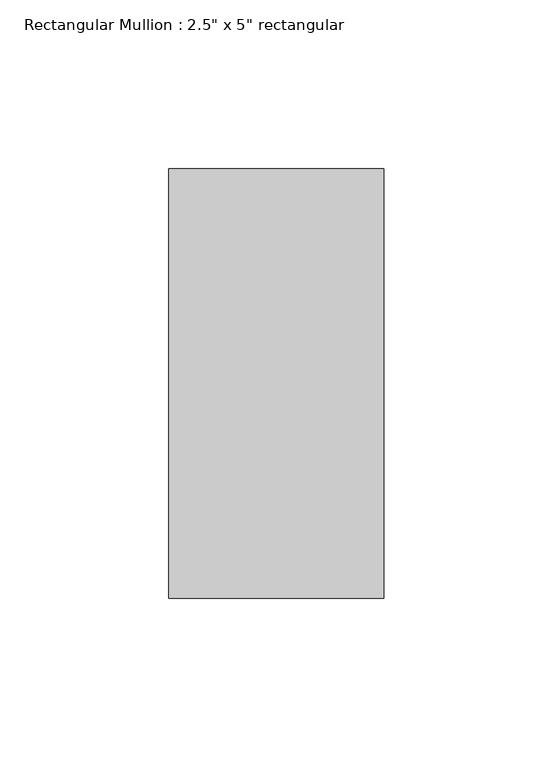
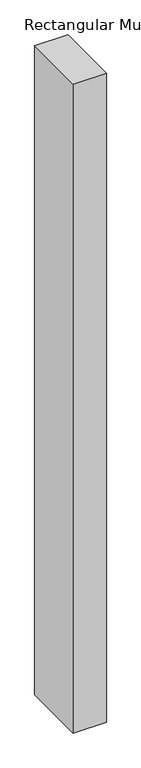
"""IFC4 building model written with IfcOpenShell, lengths in millimetres: member geometry."""

from ifc_helpers import new_model, si_unit, frame, origin, place, context, project, spatial, polyline, outline, extrude, source, transform, mapped, element, save


def member_c0a82454(model_context):
    return source(origin(), model_context, "Body", "SweptSolid", [
        extrude(outline(polyline([(0.0, 63.5), (0.0, -63.5), (-63.5, -63.5), (-63.5, 63.5), (0.0, 63.5)])), frame((0.0, 0.0, -1310.2166668), z_axis=(0.0, 0.0, 1.0), x_axis=(1.0, 0.0, 0.0)), (0.0, 0.0, 1.0), 1310.2166668),
    ])


if __name__ == "__main__":
    model = new_model("IFC4")
    model_context = context("Model", 3, world=origin())
    ifc_project = project(units=[si_unit("LENGTHUNIT", "METRE", prefix="MILLI")], contexts=[model_context])
    site = spatial("IfcSite", under=ifc_project)
    building = spatial("IfcBuilding", under=site)
    placement = place(None, origin())
    member_shape = member_c0a82454(model_context)
    element("IfcMember", 1, ObjectType="Rectangular Mullion : 2.5\" x 5\" rectangular", at=placement, inside=building, context=model_context, shape_type="MappedRepresentation", body=[
        mapped(member_shape, transform((0.0, 0.0, 0.0), x_axis=(1.0, 0.0, 0.0), y_axis=(0.0, 1.0, 0.0), z_axis=(0.0, 0.0, 1.0))),
    ])
    save(model, "model.ifc")

# Revit data of these elements
# Type "Rectangular Mullion : 2.5\" x 5\" rectangular"
#   built-in parameter 1007304 = 0.416667 (stored number, unit not read)
#   built-in parameter 1007301 = 0.104167 (stored number, unit not read)
#   built-in parameter 1007300 = 0.104167 (stored number, unit not read)
# Element 1 (IfcMember, "Rectangular Mullion : 2.5\" x 5\" rectangular")
#   Materials on its faces: "Aluminum"
# Materials
#   "Aluminum": class "Metal", colour RGB 247 247 247, transparency 0, Description = "Aluminum 6061", Cost = 0
